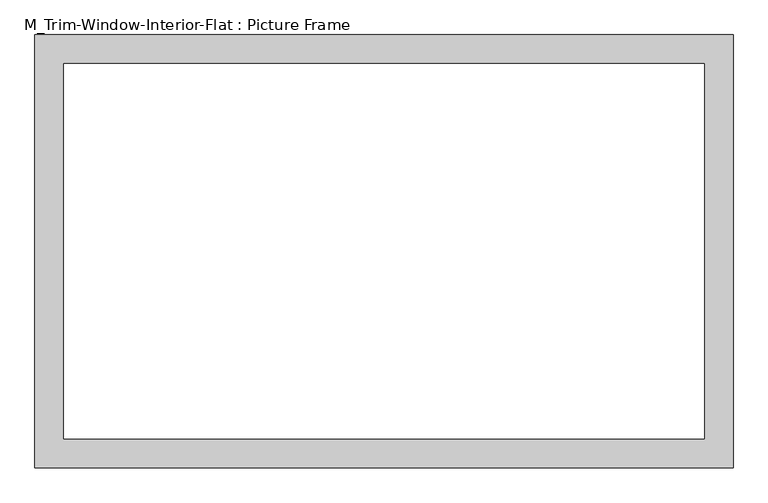
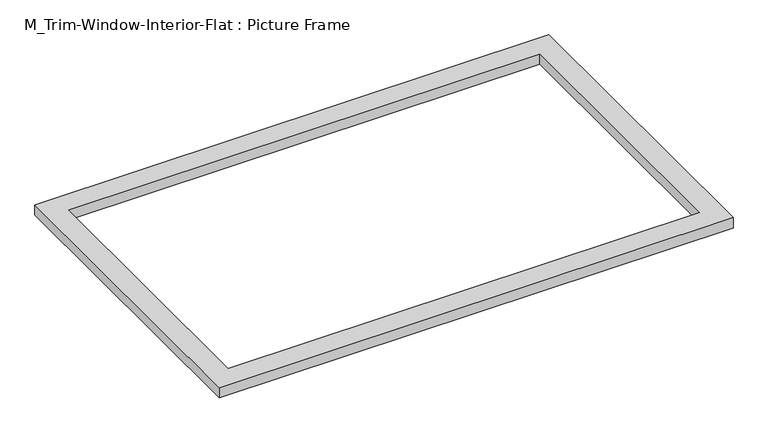
"""IFC4 building model written with IfcOpenShell, lengths in millimetres: proxy geometry, M_Trim-Window-Interior-Flat : Picture Frame."""

from ifc_helpers import new_model, si_unit, origin, origin_with_axes, place, context, project, spatial, polyline, outline, extrude, source, transform, mapped, element, save


def m_trim_window_interior_flat_picture_frame_c139440e(model_context):
    return source(origin(), model_context, "Body", "SweptSolid", [
        extrude(outline(polyline([(720.4, 47.3), (720.4, -847.3), (-720.4, -847.3), (-720.4, 47.3), (720.4, 47.3)]), holes=[polyline([(660.4, -12.7), (-660.4, -12.7), (-660.4, -787.3), (660.4, -787.3), (660.4, -12.7)])]), origin_with_axes(), (0.0, 0.0, 1.0), 30.0),
    ])


if __name__ == "__main__":
    model = new_model("IFC4")
    model_context = context("Model", 3, world=origin())
    ifc_project = project(units=[si_unit("LENGTHUNIT", "METRE", prefix="MILLI")], contexts=[model_context])
    site = spatial("IfcSite", under=ifc_project)
    building = spatial("IfcBuilding", under=site)
    placement = place(None, origin())
    m_trim_window_interior_flat_picture_frame_shape = m_trim_window_interior_flat_picture_frame_c139440e(model_context)
    element("IfcBuildingElementProxy", 1, Name="M_Trim-Window-Interior-Flat : Picture Frame", ObjectType="M_Trim-Window-Interior-Flat : Picture Frame", at=placement, inside=building, context=model_context, shape_type="MappedRepresentation", body=[
        mapped(m_trim_window_interior_flat_picture_frame_shape, transform((0.0, 0.0, 0.0), x_axis=(1.0, 0.0, 0.0), y_axis=(0.0, 1.0, 0.0), z_axis=(0.0, 0.0, 1.0))),
    ])
    save(model, "model.ifc")

# Revit data of these elements
# Type "M_Trim-Window-Interior-Flat : Picture Frame"
#   Trim Thickness_Picture Frame = 0' - 1.1811"
#   Trim Width = 0' - 2.3622"
#   Trim Thickness_with Sill = 0' - 0.7874"
#   Sill Thickness = 0' - 1.1811"
#   Opening Width [instance default] = 1' - 11.62205"
#   Opening Height [instance default] = 2' - 11.43307"
#   Default Elevation = 3' - 11.24409"
#   Sill = no
#   Picture Frame = yes
#   Trim Material [instance default] = none
# Element 1 (IfcBuildingElementProxy, "M_Trim-Window-Interior-Flat : Picture Frame")
#   Opening Width = 4' - 5"
#   Opening Height = 2' - 7.49606"
#   Trim Material = Wood - Stained
#   Materials on its faces: "Wood - Stained"
# Materials
#   "Wood - Stained": class "Wood", colour RGB 227 170 128, transparency 0, Cost = 0
